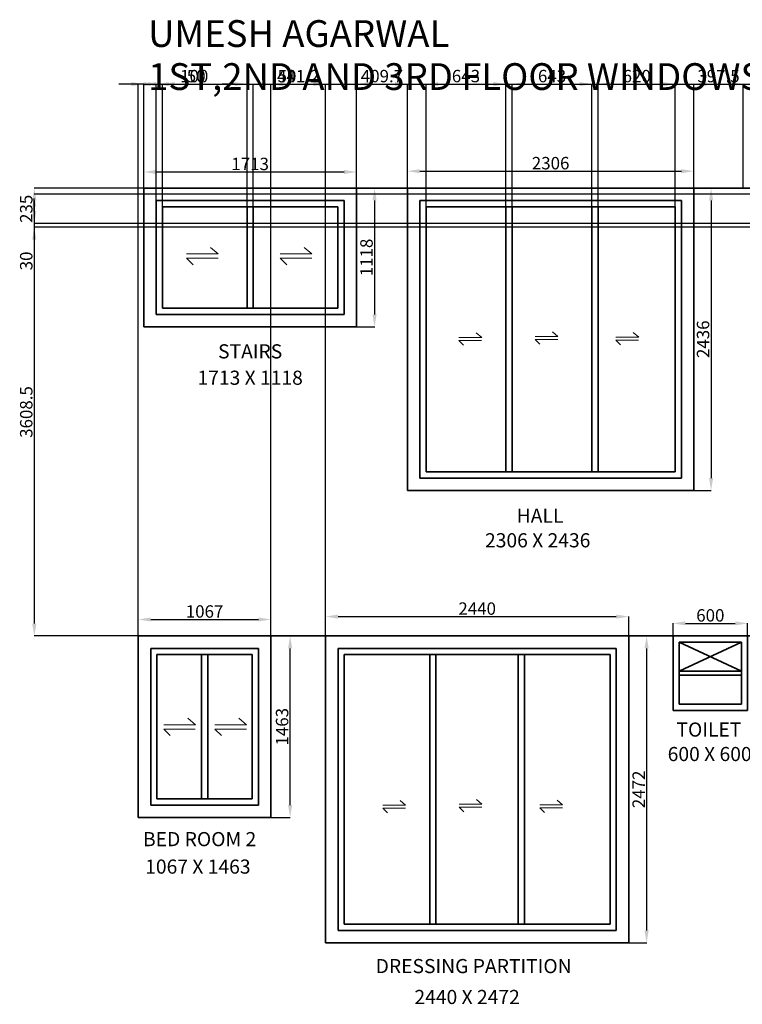
# Model space of a CAD drawing. Units: millimetres. Extents: x 5977 to 24120, y -1732 to 6209.
# Tile 1 of 3: x 5977 to 11795, y -1724 to 6209. Entities that reach past the tile are written whole.
import ezdxf

# ---------------------------------------------------------------- set-up
doc = ezdxf.new("R2010")
doc.units = ezdxf.units.MM
for name, color, linetype, lineweight in [('A-ANNO-DIMS', 2, 'Continuous', 18), ('A-ANNO-SYMB', 143, 'Continuous', 18), ('A-ANNO-TEXT', 7, 'Continuous', 25), ('A-GLAZ', 4, 'Continuous', 35)]:
    doc.layers.add(name, color=color, linetype=linetype, lineweight=lineweight)
doc.styles.get("Standard").update_dxf_attribs({"font": 'arial.ttf'})
doc.dimstyles.new('ISO-25', dxfattribs={"dimtxt": 100, "dimasz": 100, "dimexe": 1.25, "dimexo": 0.625, "dimtad": 1, "dimtxsty": 'Standard', "dimcen": 2.5, "dimadec": 0, "dimazin": 0, "dimtfac": 1, "dimtmove": 0, "dimatfit": 3, "dimfxl": 1, "dimarcsym": 0})

# ---------------------------------------------------------------- blocks, each defined once
blk = doc.blocks.new('*D1')
at = {"layer": 'A-ANNO-DIMS', "color": 0, "lineweight": -2, "transparency": 16777216}
for p, q in [((6975.8, 4852.8), (6975.8, 4983.1)), ((7075.8, 4981.9), (8588.8, 4981.9)), ((8688.8, 4852.8), (8688.8, 4983.1))]:
    blk.add_line(p, q, dxfattribs=at)
at = {"layer": 'A-ANNO-DIMS', "color": 0, "transparency": 16777216}
for points in [[(7075.8, 4998.5), (7075.8, 4965.2), (6975.8, 4981.9)], [(8588.8, 4998.5), (8588.8, 4965.2), (8688.8, 4981.9)]]:
    blk.add_solid(points, dxfattribs=at)
at = {"layer": 'Defpoints', "color": 0, "transparency": 16777216}
for p in [(8688.8, 4981.9), (6975.8, 4852.2), (8688.8, 4852.2)]:
    blk.add_point(p, dxfattribs=at)
at = {"layer": 'A-ANNO-DIMS', "color": 0, "transparency": 16777216, "insert": (7832.3, 5033.6), "char_height": 100, "attachment_point": 5}
blk.add_mtext('1713', dxfattribs=at)
blk = doc.blocks.new('*D2')
at = {"layer": 'A-ANNO-DIMS', "color": 0, "lineweight": -2, "transparency": 16777216}
for p, q in [((8689.4, 4852.2), (8835.1, 4852.2)), ((8833.9, 4752.2), (8833.9, 3834.2)), ((8689.4, 3734.2), (8835.1, 3734.2))]:
    blk.add_line(p, q, dxfattribs=at)
at = {"layer": 'A-ANNO-DIMS', "color": 0, "transparency": 16777216}
for points in [[(8817.2, 4752.2), (8850.5, 4752.2), (8833.9, 4852.2)], [(8817.2, 3834.2), (8850.5, 3834.2), (8833.9, 3734.2)]]:
    blk.add_solid(points, dxfattribs=at)
at = {"layer": 'Defpoints', "color": 0, "transparency": 16777216}
for p in [(8688.8, 4852.2), (8688.8, 3734.2), (8833.9, 3734.2)]:
    blk.add_point(p, dxfattribs=at)
at = {"layer": 'A-ANNO-DIMS', "color": 0, "transparency": 16777216, "insert": (8782.2, 4293.2), "char_height": 100, "attachment_point": 5, "rotation": 90}
blk.add_mtext('1118', dxfattribs=at)
blk = doc.blocks.new('*D3')
at = {"layer": 'A-ANNO-DIMS', "color": 0, "lineweight": -2, "transparency": 16777216}
for p, q in [((9098.5, 4852.8), (9098.5, 4989.4)), ((9198.5, 4988.2), (11304.5, 4988.2)), ((11404.5, 4852.8), (11404.5, 4989.4))]:
    blk.add_line(p, q, dxfattribs=at)
at = {"layer": 'A-ANNO-DIMS', "color": 0, "transparency": 16777216}
for points in [[(9198.5, 5004.8), (9198.5, 4971.5), (9098.5, 4988.2)], [(11304.5, 5004.8), (11304.5, 4971.5), (11404.5, 4988.2)]]:
    blk.add_solid(points, dxfattribs=at)
at = {"layer": 'Defpoints', "color": 0, "transparency": 16777216}
for p in [(11404.5, 4988.2), (9098.5, 4852.2), (11404.5, 4852.2)]:
    blk.add_point(p, dxfattribs=at)
at = {"layer": 'A-ANNO-DIMS', "color": 0, "transparency": 16777216, "insert": (10251.5, 5039.9), "char_height": 100, "attachment_point": 5}
blk.add_mtext('2306', dxfattribs=at)
blk = doc.blocks.new('*D4')
at = {"layer": 'A-ANNO-DIMS', "color": 0, "lineweight": -2, "transparency": 16777216}
for p, q in [((11405.1, 4852.2), (11544.6, 4852.2)), ((11543.4, 4752.2), (11543.4, 2516.2)), ((11405.1, 2416.2), (11544.6, 2416.2))]:
    blk.add_line(p, q, dxfattribs=at)
at = {"layer": 'A-ANNO-DIMS', "color": 0, "transparency": 16777216}
for points in [[(11526.7, 4752.2), (11560, 4752.2), (11543.4, 4852.2)], [(11526.7, 2516.2), (11560, 2516.2), (11543.4, 2416.2)]]:
    blk.add_solid(points, dxfattribs=at)
at = {"layer": 'Defpoints', "color": 0, "transparency": 16777216}
for p in [(11404.5, 4852.2), (11404.5, 2416.2), (11543.4, 2416.2)]:
    blk.add_point(p, dxfattribs=at)
at = {"layer": 'A-ANNO-DIMS', "color": 0, "transparency": 16777216, "insert": (11491.7, 3634.2), "char_height": 100, "attachment_point": 5, "rotation": 90}
blk.add_mtext('2436', dxfattribs=at)
blk = doc.blocks.new('*D21')
at = {"layer": 'A-ANNO-DIMS', "color": 0, "lineweight": -2, "transparency": 16777216}
for p, q in [((6931.9, 1244.3), (6931.9, 1377.5)), ((7031.9, 1376.2), (7898.9, 1376.2)), ((7998.9, 1244.3), (7998.9, 1377.5))]:
    blk.add_line(p, q, dxfattribs=at)
at = {"layer": 'A-ANNO-DIMS', "color": 0, "transparency": 16777216}
for points in [[(7031.9, 1392.9), (7031.9, 1359.6), (6931.9, 1376.2)], [(7898.9, 1392.9), (7898.9, 1359.6), (7998.9, 1376.2)]]:
    blk.add_solid(points, dxfattribs=at)
at = {"layer": 'Defpoints', "color": 0, "transparency": 16777216}
for p in [(7998.9, 1376.2), (6931.9, 1243.7), (7998.9, 1243.7)]:
    blk.add_point(p, dxfattribs=at)
at = {"layer": 'A-ANNO-DIMS', "color": 0, "transparency": 16777216, "insert": (7465.4, 1427.9), "char_height": 100, "attachment_point": 5}
blk.add_mtext('1067', dxfattribs=at)
blk = doc.blocks.new('*D22')
at = {"layer": 'A-ANNO-DIMS', "color": 0, "lineweight": -2, "transparency": 16777216}
for p, q in [((7999.6, 1243.7), (8155.6, 1243.7)), ((8154.3, -119.3), (8154.3, 1143.7)), ((7999.6, -219.3), (8155.6, -219.3))]:
    blk.add_line(p, q, dxfattribs=at)
at = {"layer": 'A-ANNO-DIMS', "color": 0, "transparency": 16777216}
for points in [[(8137.6, 1143.7), (8171, 1143.7), (8154.3, 1243.7)], [(8137.6, -119.3), (8171, -119.3), (8154.3, -219.3)]]:
    blk.add_solid(points, dxfattribs=at)
at = {"layer": 'Defpoints', "color": 0, "transparency": 16777216}
for p in [(7998.9, 1243.7), (8154.3, 1243.7), (7998.9, -219.3)]:
    blk.add_point(p, dxfattribs=at)
at = {"layer": 'A-ANNO-DIMS', "color": 0, "transparency": 16777216, "insert": (8102.6, 512.2), "char_height": 100, "attachment_point": 5, "rotation": 90}
blk.add_mtext('1463', dxfattribs=at)
blk = doc.blocks.new('*D23')
at = {"layer": 'A-ANNO-DIMS', "color": 0, "lineweight": -2, "transparency": 16777216}
for p, q in [((8440.1, 1244.3), (8440.1, 1400.7)), ((8540.1, 1399.4), (10780.1, 1399.4)), ((10880.1, 1244.3), (10880.1, 1400.7))]:
    blk.add_line(p, q, dxfattribs=at)
at = {"layer": 'A-ANNO-DIMS', "color": 0, "transparency": 16777216}
for points in [[(8540.1, 1416.1), (8540.1, 1382.7), (8440.1, 1399.4)], [(10780.1, 1416.1), (10780.1, 1382.7), (10880.1, 1399.4)]]:
    blk.add_solid(points, dxfattribs=at)
at = {"layer": 'Defpoints', "color": 0, "transparency": 16777216}
for p in [(10880.1, 1399.4), (8440.1, 1243.7), (10880.1, 1243.7)]:
    blk.add_point(p, dxfattribs=at)
at = {"layer": 'A-ANNO-DIMS', "color": 0, "transparency": 16777216, "insert": (9660.1, 1451.1), "char_height": 100, "attachment_point": 5}
blk.add_mtext('2440', dxfattribs=at)
blk = doc.blocks.new('*D24')
at = {"layer": 'A-ANNO-DIMS', "color": 0, "lineweight": -2, "transparency": 16777216}
for p, q in [((10880.7, 1243.7), (11025.5, 1243.7)), ((11024.2, 1143.7), (11024.2, -1128.3)), ((10880.7, -1228.3), (11025.5, -1228.3))]:
    blk.add_line(p, q, dxfattribs=at)
at = {"layer": 'A-ANNO-DIMS', "color": 0, "transparency": 16777216}
for points in [[(11007.5, 1143.7), (11040.9, 1143.7), (11024.2, 1243.7)], [(11007.5, -1128.3), (11040.9, -1128.3), (11024.2, -1228.3)]]:
    blk.add_solid(points, dxfattribs=at)
at = {"layer": 'Defpoints', "color": 0, "transparency": 16777216}
for p in [(10880.1, 1243.7), (10880.1, -1228.3), (11024.2, -1228.3)]:
    blk.add_point(p, dxfattribs=at)
at = {"layer": 'A-ANNO-DIMS', "color": 0, "transparency": 16777216, "insert": (10973.4, 7.7), "char_height": 100, "attachment_point": 5, "rotation": 90}
blk.add_mtext('2472', dxfattribs=at)
blk = doc.blocks.new('*D27')
at = {"layer": 'A-ANNO-DIMS', "color": 0, "lineweight": -2, "transparency": 16777216}
for p, q in [((11237.4, 1244.3), (11237.4, 1346.1)), ((11337.4, 1344.9), (11737.4, 1344.9)), ((11837.4, 1244.3), (11837.4, 1346.1))]:
    blk.add_line(p, q, dxfattribs=at)
at = {"layer": 'A-ANNO-DIMS', "color": 0, "transparency": 16777216}
for points in [[(11337.4, 1361.5), (11337.4, 1328.2), (11237.4, 1344.9)], [(11737.4, 1361.5), (11737.4, 1328.2), (11837.4, 1344.9)]]:
    blk.add_solid(points, dxfattribs=at)
at = {"layer": 'Defpoints', "color": 0, "transparency": 16777216}
for p in [(11837.4, 1344.9), (11237.4, 1243.7), (11837.4, 1243.7)]:
    blk.add_point(p, dxfattribs=at)
at = {"layer": 'A-ANNO-DIMS', "color": 0, "transparency": 16777216, "insert": (11537.4, 1396.6), "char_height": 100, "attachment_point": 5}
blk.add_mtext('600', dxfattribs=at)
blk = doc.blocks.new('WIN-600x600-TOILET')
for p, q in [((16540.9, 4852.2), (16540.9, 4252.2)), ((17140.9, 4252.2), (17140.9, 4852.2)), ((16590.9, 4802.2), (16590.9, 4302.2)), ((16590.9, 4802.2), (17090.9, 4802.2)), ((16590.9, 4567.2), (17090.9, 4802.2)), ((17090.9, 4567.2), (16590.9, 4802.2)), ((17090.9, 4302.2), (17090.9, 4802.2)), ((16590.9, 4567.2), (17090.9, 4567.2)), ((16590.9, 4302.2), (17090.9, 4302.2)), ((16540.9, 4252.2), (17140.9, 4252.2))]:
    blk.add_line(p, q)
blk = doc.blocks.new('ARROW-SLIDE')
for p, q in [((14721.8, 21.3), (14904.6, 21.3)), ((14904.6, 21.3), (14860.5, 58.6)), ((14721.8, -3.8), (14904.1, -3.8)), ((14721.8, -3.8), (14759.4, -41.4))]:
    blk.add_line(p, q)
blk = doc.blocks.new('ARROW-SLIDE-LG')
for p, q in [((7575.1, 4322.2), (7513.8, 4374)), ((7321, 4287.2), (7574.5, 4287.2)), ((7321, 4287.2), (7373.4, 4234.9)), ((7321.1, 4322.2), (7575.1, 4322.2))]:
    blk.add_line(p, q)
blk = doc.blocks.new('*D41')
at = {"layer": 'A-ANNO-DIMS', "color": 0, "lineweight": -2, "transparency": 16777216}
for p, q in [((6975.8, 4852.8), (6975.8, 5690.9)), ((7075.8, 5689.7), (23502.6, 5689.7)), ((23602.6, 4852.8), (23602.6, 5690.9))]:
    blk.add_line(p, q, dxfattribs=at)
at = {"layer": 'A-ANNO-DIMS', "color": 0, "transparency": 16777216}
for points in [[(7075.8, 5706.3), (7075.8, 5673), (6975.8, 5689.7)], [(23502.6, 5706.3), (23502.6, 5673), (23602.6, 5689.7)]]:
    blk.add_solid(points, dxfattribs=at)
at = {"layer": 'Defpoints', "color": 0, "transparency": 16777216}
for p in [(23602.6, 5689.7), (6975.8, 4852.2), (23602.6, 4852.2)]:
    blk.add_point(p, dxfattribs=at)
at = {"layer": 'A-ANNO-DIMS', "color": 0, "transparency": 16777216, "insert": (15289.2, 5741.3), "char_height": 100, "attachment_point": 5}
blk.add_mtext('16627', dxfattribs=at)
blk = doc.blocks.new('*D42')
at = {"layer": 'A-ANNO-DIMS', "color": 0, "lineweight": -2, "transparency": 16777216}
for p, q in [((6931.9, 1244.3), (6931.9, 5690.9)), ((7031.9, 5689.7), (20409.7, 5689.7)), ((20509.7, 1244.3), (20509.7, 5690.9))]:
    blk.add_line(p, q, dxfattribs=at)
at = {"layer": 'A-ANNO-DIMS', "color": 0, "transparency": 16777216}
for points in [[(7031.9, 5706.3), (7031.9, 5673), (6931.9, 5689.7)], [(20409.7, 5706.3), (20409.7, 5673), (20509.7, 5689.7)]]:
    blk.add_solid(points, dxfattribs=at)
at = {"layer": 'Defpoints', "color": 0, "transparency": 16777216}
for p in [(20509.7, 5689.7), (6931.9, 1243.7), (20509.7, 1243.7)]:
    blk.add_point(p, dxfattribs=at)
at = {"layer": 'A-ANNO-DIMS', "color": 0, "transparency": 16777216, "insert": (13720.8, 5741.4), "char_height": 100, "attachment_point": 5}
blk.add_mtext('13578', dxfattribs=at)
blk = doc.blocks.new('*D43')
at = {"layer": 'A-ANNO-DIMS', "color": 0, "lineweight": -2, "transparency": 16777216}
for p, q in [((6975.1, 4852.2), (6093.2, 4852.2)), ((6094.4, 4752.2), (6094.4, 1343.7)), ((6931.3, 1243.7), (6093.2, 1243.7))]:
    blk.add_line(p, q, dxfattribs=at)
at = {"layer": 'A-ANNO-DIMS', "color": 0, "transparency": 16777216}
for points in [[(6077.8, 4752.2), (6111.1, 4752.2), (6094.4, 4852.2)], [(6077.8, 1343.7), (6111.1, 1343.7), (6094.4, 1243.7)]]:
    blk.add_solid(points, dxfattribs=at)
at = {"layer": 'Defpoints', "color": 0, "transparency": 16777216}
for p in [(6975.8, 4852.2), (6094.4, 1243.7), (6931.9, 1243.7)]:
    blk.add_point(p, dxfattribs=at)
at = {"layer": 'A-ANNO-DIMS', "color": 0, "transparency": 16777216, "insert": (6042.7, 3047.9), "char_height": 100, "attachment_point": 5, "rotation": 90}
blk.add_mtext('3608.5', dxfattribs=at)
blk = doc.blocks.new('*D44')
at = {"layer": 'A-ANNO-DIMS', "color": 0, "lineweight": -2, "transparency": 16777216}
for p, q in [((8688.8, 4852.8), (8688.8, 5690.9)), ((8788.8, 5689.7), (8998.5, 5689.7)), ((9098.5, 4852.8), (9098.5, 5690.9))]:
    blk.add_line(p, q, dxfattribs=at)
at = {"layer": 'A-ANNO-DIMS', "color": 0, "transparency": 16777216}
for points in [[(8788.8, 5706.3), (8788.8, 5673), (8688.8, 5689.7)], [(8998.5, 5706.3), (8998.5, 5673), (9098.5, 5689.7)]]:
    blk.add_solid(points, dxfattribs=at)
at = {"layer": 'Defpoints', "color": 0, "transparency": 16777216}
for p in [(9098.5, 5689.7), (8688.8, 4852.2), (9098.5, 4852.2)]:
    blk.add_point(p, dxfattribs=at)
at = {"layer": 'A-ANNO-DIMS', "color": 0, "transparency": 16777216, "insert": (8893.6, 5741.3), "char_height": 100, "attachment_point": 5}
blk.add_mtext('409.7', dxfattribs=at)
blk = doc.blocks.new('*D45')
at = {"layer": 'A-ANNO-DIMS', "color": 0, "lineweight": -2, "transparency": 16777216}
for p, q in [((11404.5, 4852.8), (11404.5, 5690.9)), ((11504.5, 5689.7), (11702, 5689.7)), ((11802, 4852.8), (11802, 5690.9))]:
    blk.add_line(p, q, dxfattribs=at)
at = {"layer": 'A-ANNO-DIMS', "color": 0, "transparency": 16777216}
for points in [[(11504.5, 5706.3), (11504.5, 5673), (11404.5, 5689.7)], [(11702, 5706.3), (11702, 5673), (11802, 5689.7)]]:
    blk.add_solid(points, dxfattribs=at)
at = {"layer": 'Defpoints', "color": 0, "transparency": 16777216}
for p in [(11802, 5689.7), (11404.5, 4852.2), (11802, 4852.2)]:
    blk.add_point(p, dxfattribs=at)
at = {"layer": 'A-ANNO-DIMS', "color": 0, "transparency": 16777216, "insert": (11603.2, 5741.4), "char_height": 100, "attachment_point": 5}
blk.add_mtext('397.5', dxfattribs=at)
blk = doc.blocks.new('*D54')
at = {"layer": 'A-ANNO-DIMS', "color": 0, "lineweight": -2, "transparency": 16777216}
for p, q in [((7998.9, 1244.3), (7998.9, 5690.9)), ((8098.9, 5689.7), (8340.1, 5689.7)), ((8440.1, 1244.3), (8440.1, 5690.9))]:
    blk.add_line(p, q, dxfattribs=at)
at = {"layer": 'A-ANNO-DIMS', "color": 0, "transparency": 16777216}
for points in [[(8098.9, 5706.3), (8098.9, 5673), (7998.9, 5689.7)], [(8340.1, 5706.3), (8340.1, 5673), (8440.1, 5689.7)]]:
    blk.add_solid(points, dxfattribs=at)
at = {"layer": 'Defpoints', "color": 0, "transparency": 16777216}
for p in [(8440.1, 5689.7), (7998.9, 1243.7), (8440.1, 1243.7)]:
    blk.add_point(p, dxfattribs=at)
at = {"layer": 'A-ANNO-DIMS', "color": 0, "transparency": 16777216, "insert": (8219.5, 5740.5), "char_height": 100, "attachment_point": 5}
blk.add_mtext('441.2', dxfattribs=at)
blk = doc.blocks.new('*D61')
at = {"layer": 'A-ANNO-DIMS', "color": 0, "lineweight": -2, "transparency": 16777216}
for p, q in [((6875.8, 5689.7), (6775.8, 5689.7)), ((6975.8, 4852.8), (6975.8, 5690.9)), ((6975.8, 5689.7), (7075.8, 5689.7)), ((7075.8, 4752.8), (7075.8, 5690.9)), ((7175.8, 5689.7), (7488.2, 5689.7))]:
    blk.add_line(p, q, dxfattribs=at)
at = {"layer": 'A-ANNO-DIMS', "color": 0, "transparency": 16777216}
for points in [[(6875.8, 5706.3), (6875.8, 5673), (6975.8, 5689.7)], [(7175.8, 5706.3), (7175.8, 5673), (7075.8, 5689.7)]]:
    blk.add_solid(points, dxfattribs=at)
at = {"layer": 'Defpoints', "color": 0, "transparency": 16777216}
for p in [(7075.8, 5689.7), (6975.8, 4852.2), (7075.8, 4752.2)]:
    blk.add_point(p, dxfattribs=at)
at = {"layer": 'A-ANNO-DIMS', "color": 0, "transparency": 16777216, "insert": (7382, 5741.3), "char_height": 100, "attachment_point": 5}
blk.add_mtext('100', dxfattribs=at)
blk = doc.blocks.new('*D62')
at = {"layer": 'A-ANNO-DIMS', "color": 0, "lineweight": -2, "transparency": 16777216}
for p, q in [((6975.8, 5689.7), (6875.8, 5689.7)), ((7075.8, 4752.8), (7075.8, 5690.9)), ((7075.8, 5689.7), (7125.8, 5689.7)), ((7125.8, 4702.8), (7125.8, 5690.9)), ((7225.8, 5689.7), (7469.9, 5689.7))]:
    blk.add_line(p, q, dxfattribs=at)
at = {"layer": 'A-ANNO-DIMS', "color": 0, "transparency": 16777216}
for points in [[(6975.8, 5706.3), (6975.8, 5673), (7075.8, 5689.7)], [(7225.8, 5706.3), (7225.8, 5673), (7125.8, 5689.7)]]:
    blk.add_solid(points, dxfattribs=at)
at = {"layer": 'Defpoints', "color": 0, "transparency": 16777216}
for p in [(7125.8, 5689.7), (7075.8, 4752.2), (7125.8, 4702.2)]:
    blk.add_point(p, dxfattribs=at)
at = {"layer": 'A-ANNO-DIMS', "color": 0, "transparency": 16777216, "insert": (7397.8, 5741.3), "char_height": 100, "attachment_point": 5}
blk.add_mtext('50', dxfattribs=at)
blk = doc.blocks.new('*D63')
at = {"layer": 'A-ANNO-DIMS', "color": 0, "lineweight": -2, "transparency": 16777216}
for p, q in [((7707.3, 5689.7), (7607.3, 5689.7)), ((7807.3, 4702.8), (7807.3, 5690.9)), ((7807.3, 5689.7), (7857.3, 5689.7)), ((7857.3, 4702.8), (7857.3, 5690.9)), ((7957.3, 5689.7), (8201.4, 5689.7))]:
    blk.add_line(p, q, dxfattribs=at)
at = {"layer": 'A-ANNO-DIMS', "color": 0, "transparency": 16777216}
for points in [[(7707.3, 5706.3), (7707.3, 5673), (7807.3, 5689.7)], [(7957.3, 5706.3), (7957.3, 5673), (7857.3, 5689.7)]]:
    blk.add_solid(points, dxfattribs=at)
at = {"layer": 'Defpoints', "color": 0, "transparency": 16777216}
for p in [(7857.3, 5689.7), (7807.3, 4702.2), (7857.3, 4702.2)]:
    blk.add_point(p, dxfattribs=at)
at = {"layer": 'A-ANNO-DIMS', "color": 0, "transparency": 16777216, "insert": (8129.3, 5741.3), "char_height": 100, "attachment_point": 5}
blk.add_mtext('50', dxfattribs=at)
blk = doc.blocks.new('*D64')
at = {"layer": 'A-ANNO-DIMS', "color": 0, "lineweight": -2, "transparency": 16777216}
for p, q in [((9248.5, 4702.8), (9248.5, 5690.9)), ((9348.5, 5689.7), (9791.5, 5689.7)), ((9891.5, 4702.8), (9891.5, 5690.9))]:
    blk.add_line(p, q, dxfattribs=at)
at = {"layer": 'A-ANNO-DIMS', "color": 0, "transparency": 16777216}
for points in [[(9348.5, 5706.3), (9348.5, 5673), (9248.5, 5689.7)], [(9791.5, 5706.3), (9791.5, 5673), (9891.5, 5689.7)]]:
    blk.add_solid(points, dxfattribs=at)
at = {"layer": 'Defpoints', "color": 0, "transparency": 16777216}
for p in [(9891.5, 5689.7), (9248.5, 4702.2), (9891.5, 4702.2)]:
    blk.add_point(p, dxfattribs=at)
at = {"layer": 'A-ANNO-DIMS', "color": 0, "transparency": 16777216, "insert": (9570, 5741.4), "char_height": 100, "attachment_point": 5}
blk.add_mtext('643', dxfattribs=at)
blk = doc.blocks.new('*D65')
at = {"layer": 'A-ANNO-DIMS', "color": 0, "lineweight": -2, "transparency": 16777216}
for p, q in [((9941.5, 4702.8), (9941.5, 5690.9)), ((10041.5, 5689.7), (10484.5, 5689.7)), ((10584.5, 4702.8), (10584.5, 5690.9))]:
    blk.add_line(p, q, dxfattribs=at)
at = {"layer": 'A-ANNO-DIMS', "color": 0, "transparency": 16777216}
for points in [[(10041.5, 5706.3), (10041.5, 5673), (9941.5, 5689.7)], [(10484.5, 5706.3), (10484.5, 5673), (10584.5, 5689.7)]]:
    blk.add_solid(points, dxfattribs=at)
at = {"layer": 'Defpoints', "color": 0, "transparency": 16777216}
for p in [(10584.5, 5689.7), (9941.5, 4702.2), (10584.5, 4702.2)]:
    blk.add_point(p, dxfattribs=at)
at = {"layer": 'A-ANNO-DIMS', "color": 0, "transparency": 16777216, "insert": (10263, 5741.4), "char_height": 100, "attachment_point": 5}
blk.add_mtext('643', dxfattribs=at)
blk = doc.blocks.new('*D66')
at = {"layer": 'A-ANNO-DIMS', "color": 0, "lineweight": -2, "transparency": 16777216}
for p, q in [((10634.5, 4702.8), (10634.5, 5690.9)), ((10734.5, 5689.7), (11154.5, 5689.7)), ((11254.5, 4702.8), (11254.5, 5690.9))]:
    blk.add_line(p, q, dxfattribs=at)
at = {"layer": 'A-ANNO-DIMS', "color": 0, "transparency": 16777216}
for points in [[(10734.5, 5706.3), (10734.5, 5673), (10634.5, 5689.7)], [(11154.5, 5706.3), (11154.5, 5673), (11254.5, 5689.7)]]:
    blk.add_solid(points, dxfattribs=at)
at = {"layer": 'Defpoints', "color": 0, "transparency": 16777216}
for p in [(11254.5, 5689.7), (10634.5, 4702.2), (11254.5, 4702.2)]:
    blk.add_point(p, dxfattribs=at)
at = {"layer": 'A-ANNO-DIMS', "color": 0, "transparency": 16777216, "insert": (10944.5, 5741.3), "char_height": 100, "attachment_point": 5}
blk.add_mtext('620', dxfattribs=at)
blk = doc.blocks.new('*D67')
at = {"layer": 'A-ANNO-DIMS', "color": 0, "lineweight": -2, "transparency": 16777216}
for p, q in [((16590.3, 4802.2), (6093.2, 4802.2)), ((6094.4, 4702.2), (6094.4, 4667.2)), ((16590.3, 4567.2), (6093.2, 4567.2))]:
    blk.add_line(p, q, dxfattribs=at)
at = {"layer": 'A-ANNO-DIMS', "color": 0, "transparency": 16777216}
for points in [[(6077.8, 4702.2), (6111.1, 4702.2), (6094.4, 4802.2)], [(6077.8, 4667.2), (6111.1, 4667.2), (6094.4, 4567.2)]]:
    blk.add_solid(points, dxfattribs=at)
at = {"layer": 'Defpoints', "color": 0, "transparency": 16777216}
for p in [(16590.9, 4802.2), (6094.4, 4567.2), (16590.9, 4567.2)]:
    blk.add_point(p, dxfattribs=at)
at = {"layer": 'A-ANNO-DIMS', "color": 0, "transparency": 16777216, "insert": (6042.7, 4684.7), "char_height": 100, "attachment_point": 5, "rotation": 90}
blk.add_mtext('235', dxfattribs=at)
blk = doc.blocks.new('*D68')
at = {"layer": 'A-ANNO-DIMS', "color": 0, "lineweight": -2, "transparency": 16777216}
for p, q in [((6094.4, 4667.2), (6094.4, 4767.2)), ((16590.3, 4567.2), (6093.2, 4567.2)), ((16590.3, 4537.2), (6093.2, 4537.2)), ((6094.4, 4567.2), (6094.4, 4537.2)), ((6094.4, 4437.2), (6094.4, 4193.1))]:
    blk.add_line(p, q, dxfattribs=at)
at = {"layer": 'A-ANNO-DIMS', "color": 0, "transparency": 16777216}
for points in [[(6077.8, 4667.2), (6111.1, 4667.2), (6094.4, 4567.2)], [(6077.8, 4437.2), (6111.1, 4437.2), (6094.4, 4537.2)]]:
    blk.add_solid(points, dxfattribs=at)
at = {"layer": 'Defpoints', "color": 0, "transparency": 16777216}
for p in [(6094.4, 4537.2), (16590.9, 4567.2), (16590.9, 4537.2)]:
    blk.add_point(p, dxfattribs=at)
at = {"layer": 'A-ANNO-DIMS', "color": 0, "transparency": 16777216, "insert": (6042.7, 4265.1), "char_height": 100, "attachment_point": 5, "rotation": 90}
blk.add_mtext('30', dxfattribs=at)

msp = doc.modelspace()

# ---------------------------------------------------------------- linework, layer by layer
at = {"layer": 'A-GLAZ'}
for p, q in [((8688.757, 4852.16), (6975.757, 4852.16)), ((6975.757, 4852.16), (6975.757, 3734.16)), ((6975.757, 4852.16), (19747.827, 4852.16)), ((8688.757, 3734.16), (8688.757, 4852.16)), ((9098.482, 4852.16), (9098.482, 2416.16)), ((11404.482, 2416.16), (11404.482, 4852.16)), ((7075.757, 4752.16), (8588.757, 4752.16)), ((7075.757, 4752.16), (7075.757, 3834.16)), ((7125.757, 4702.16), (7125.757, 3884.16)), ((7125.757, 4702.16), (8538.757, 4702.16)), ((7807.257, 4702.16), (7807.257, 3884.16)), ((7857.257, 4702.16), (7857.257, 3884.16)), ((8538.757, 3884.16), (8538.757, 4702.16)), ((8588.757, 3834.16), (8588.757, 4752.16)), ((9198.482, 4752.16), (9198.482, 2516.16)), ((9198.482, 4752.16), (11304.482, 4752.16)), ((9248.482, 4702.16), (9248.482, 2566.16)), ((9248.482, 4702.16), (11254.482, 4702.16)), ((9891.482, 4702.16), (9891.482, 2566.16)), ((9941.482, 4702.16), (9941.482, 2566.16)), ((10584.482, 4702.16), (10584.482, 2566.16)), ((10634.482, 4702.16), (10634.482, 2566.16)), ((11254.482, 2566.16), (11254.482, 4702.16)), ((11304.482, 2516.16), (11304.482, 4752.16)), ((7075.757, 3834.16), (8588.757, 3834.16)), ((7125.757, 3884.16), (8538.757, 3884.16)), ((6975.757, 3734.16), (8688.757, 3734.16)), ((9248.482, 2566.16), (11254.482, 2566.16)), ((9198.482, 2516.16), (11304.482, 2516.16)), ((9098.482, 2416.16), (11404.482, 2416.16)), ((6931.935, 1243.651), (20509.687, 1243.651)), ((6931.935, 1243.651), (6931.935, -219.349)), ((7998.935, -219.349), (7998.935, 1243.651)), ((8440.11, 1243.651), (8440.11, -1228.349)), ((10880.11, -1228.349), (10880.11, 1243.651)), ((7031.935, 1143.651), (7031.935, -119.349)), ((7031.935, 1143.651), (7898.935, 1143.651)), ((7898.935, -119.349), (7898.935, 1143.651)), ((8540.11, 1143.651), (10780.11, 1143.651)), ((8540.11, 1143.651), (8540.11, -1128.349)), ((10780.11, -1128.349), (10780.11, 1143.651)), ((7081.935, 1093.651), (7081.935, -69.349)), ((7081.935, 1093.651), (7848.935, 1093.651)), ((7440.435, -69.349), (7440.435, 1093.651)), ((7490.435, -69.349), (7490.435, 1093.651)), ((7848.935, -69.349), (7848.935, 1093.651)), ((8590.11, 1093.651), (10730.11, 1093.651)), ((8590.11, 1093.651), (8590.11, -1078.349)), ((9278.11, 1093.651), (9278.11, -1078.349)), ((9328.11, 1093.651), (9328.11, -1078.349)), ((9991.11, 1093.651), (9991.11, -1078.349)), ((10041.11, 1093.651), (10041.11, -1078.349)), ((10730.11, -1078.349), (10730.11, 1093.651)), ((11287.351, 928.651), (11787.351, 928.651)), ((7081.935, -69.349), (7848.935, -69.349)), ((7031.935, -119.349), (7898.935, -119.349)), ((6931.935, -219.349), (7998.935, -219.349)), ((8590.11, -1078.349), (10730.11, -1078.349)), ((8540.11, -1128.349), (10780.11, -1128.349)), ((8440.11, -1228.349), (10880.11, -1228.349))]:
    msp.add_line(p, q, dxfattribs=at)

# ---------------------------------------------------------------- block references
at = {"layer": 'A-ANNO-SYMB'}
for name, p in [('ARROW-SLIDE-LG', (0, 0)), ('ARROW-SLIDE-LG', (753.371, 0)), ('ARROW-SLIDE', (-5208.144, 3627.925)), ('ARROW-SLIDE', (-4594.266, 3635.135)), ('ARROW-SLIDE', (-3944.084, 3629.437)), ('ARROW-SLIDE-LG', (-183.985, -3793.877)), ('ARROW-SLIDE-LG', (227.771, -3793.877)), ('ARROW-SLIDE', (-5206.621, -132.484)), ('ARROW-SLIDE', (-5820.499, -139.693)), ('ARROW-SLIDE', (-4556.439, -138.181))]:
    msp.add_blockref(name, p, dxfattribs=at)
at = {"layer": 'A-GLAZ'}
msp.add_blockref('WIN-600x600-TOILET', (-5303.553, -3608.51), dxfattribs=at)

# ---------------------------------------------------------------- texts
at = {"layer": 'A-ANNO-TEXT'}
for s, height, p in [('UMESH AGARWAL', 215.75319, (7010.9, 5989.066)), ('1ST,2ND AND 3RD FLOOR WINDOWS', 215.75319, (7010.9, 5642.477)), ('STAIRS ', 113.8754, (7574.056, 3479.49)), ('1713 X 1118', 113.87539, (7408.339, 3267.186)), ('HALL ', 113.8754, (9978.218, 2155.241)), ('2306 X 2436', 113.87539, (9723.372, 1957.407)), ('TOILET', 113.8754, (11264.499, 432.677)), ('600 X 600', 113.8754, (11193.932, 235.504)), ('BED ROOM 2', 113.8754, (6969.814, -450.099)), ('1067 X 1463', 113.87539, (6987.347, -671.473)), ('DRESSING PARTITION', 113.87539, (8842.587, -1473.047)), ('2440 X 2472', 113.87539, (9155.016, -1722.004))]:
    msp.add_text(s, height=height, dxfattribs=at).set_placement(p)

# ---------------------------------------------------------------- dimensions: what is measured, and where the dimension line sits
at = {"layer": 'A-ANNO-DIMS'}
for base, p1, p2, override, picture, middle in [((7075.757, 5689.66), (6975.757, 4852.16), (7075.757, 4752.16), {"dimdec": 0, "dimlfac": 1, "dimrnd": 0, "dimzin": 0, "dimdsep": 46, "dimlunit": 2}, '*D61', (7381.975, 5741.343)), ((7125.757, 5689.66), (7075.757, 4752.16), (7125.757, 4702.16), {"dimdec": 0, "dimlfac": 1, "dimrnd": 0, "dimzin": 0, "dimdsep": 46, "dimlunit": 2}, '*D62', (7397.835, 5741.343)), ((20509.687, 5689.66), (6931.935, 1243.651), (20509.687, 1243.651), {"dimdec": 0, "dimlfac": 1, "dimrnd": 0, "dimzin": 0, "dimdsep": 46, "dimlunit": 2}, '*D42', (13720.811, 5741.377)), ((23602.612, 5689.66), (6975.757, 4852.16), (23602.612, 4852.16), {"dimdec": 0, "dimlfac": 1, "dimrnd": 0, "dimzin": 0, "dimdsep": 46, "dimlunit": 2}, '*D41', (15289.184, 5741.343)), ((7857.257, 5689.66), (7807.257, 4702.16), (7857.257, 4702.16), {"dimdec": 0, "dimlfac": 1, "dimrnd": 0, "dimzin": 0, "dimdsep": 46, "dimlunit": 2}, '*D63', (8129.335, 5741.343)), ((8440.11, 5689.66), (7998.935, 1243.651), (8440.11, 1243.651), {"dimdec": 1, "dimlfac": 1, "dimrnd": 0, "dimzin": 0, "dimdsep": 46, "dimlunit": 2}, '*D54', (8219.523, 5740.49)), ((9098.482, 5689.66), (8688.757, 4852.16), (9098.482, 4852.16), {"dimdec": 1, "dimlfac": 1, "dimrnd": 0, "dimzin": 0, "dimdsep": 46, "dimlunit": 2}, '*D44', (8893.619, 5741.343)), ((9891.482, 5689.66), (9248.482, 4702.16), (9891.482, 4702.16), {"dimdec": 0, "dimlfac": 1, "dimrnd": 0, "dimzin": 0, "dimdsep": 46, "dimlunit": 2}, '*D64', (9569.982, 5741.377)), ((10584.482, 5689.66), (9941.482, 4702.16), (10584.482, 4702.16), {"dimdec": 0, "dimlfac": 1, "dimrnd": 0, "dimzin": 0, "dimdsep": 46, "dimlunit": 2}, '*D65', (10262.982, 5741.377)), ((11254.482, 5689.66), (10634.482, 4702.16), (11254.482, 4702.16), {"dimdec": 0, "dimlfac": 1, "dimrnd": 0, "dimzin": 0, "dimdsep": 46, "dimlunit": 2}, '*D66', (10944.482, 5741.343)), ((11801.995, 5689.66), (11404.482, 4852.16), (11801.995, 4852.16), {"dimdec": 1, "dimlfac": 1, "dimrnd": 0, "dimzin": 0, "dimdsep": 46, "dimlunit": 2}, '*D45', (11603.238, 5741.377)), ((8688.757, 4981.878), (6975.757, 4852.16), (8688.757, 4852.16), {"dimclrd": 0, "dimclre": 0, "dimclrt": 0}, '*D1', (7832.257, 5033.594)), ((11404.482, 4988.157), (9098.482, 4852.16), (11404.482, 4852.16), {"dimclrd": 0, "dimclre": 0, "dimclrt": 0}, '*D3', (10251.482, 5039.873)), ((10880.11, 1399.407), (8440.11, 1243.651), (10880.11, 1243.651), {"dimclrd": 0, "dimclre": 0, "dimclrt": 0}, '*D23', (9660.11, 1451.089)), ((7998.935, 1376.225), (6931.935, 1243.651), (7998.935, 1243.651), {"dimclrd": 0, "dimclre": 0, "dimclrt": 0}, '*D21', (7465.435, 1427.908)), ((11837.351, 1344.88), (11237.351, 1243.651), (11837.351, 1243.651), {"dimclrd": 0, "dimclre": 0, "dimclrt": 0}, '*D27', (11537.351, 1396.562))]:
    dim = msp.add_linear_dim(base=base, p1=p1, p2=p2, dimstyle='ISO-25', override=override, dxfattribs=at)
    dim.commit()
    dim.dimension.update_dxf_attribs({"geometry": picture, "text_midpoint": middle})
for base, p1, p2, override, picture, middle in [((6094.435, 1243.651), (6975.757, 4852.16), (6931.935, 1243.651), {"dimdec": 1, "dimlfac": 1, "dimrnd": 0, "dimzin": 0, "dimdsep": 46, "dimlunit": 2}, '*D43', (6042.718, 3047.906)), ((8833.853, 3734.16), (8688.757, 4852.16), (8688.757, 3734.16), {"dimclrd": 0, "dimclre": 0, "dimclrt": 0}, '*D2', (8782.171, 4293.16)), ((11543.373, 2416.16), (11404.482, 4852.16), (11404.482, 2416.16), {"dimclrd": 0, "dimclre": 0, "dimclrt": 0}, '*D4', (11491.656, 3634.16)), ((6094.435, 4567.16), (16590.904, 4802.16), (16590.904, 4567.16), {"dimdec": 0, "dimlfac": 1, "dimrnd": 0, "dimzin": 0, "dimdsep": 46, "dimlunit": 2}, '*D67', (6042.718, 4684.66)), ((6094.435, 4537.16), (16590.904, 4567.16), (16590.904, 4537.16), {"dimdec": 0, "dimlfac": 1, "dimrnd": 0, "dimzin": 0, "dimdsep": 46, "dimlunit": 2}, '*D68', (6042.718, 4265.117)), ((8154.307, 1243.651), (7998.935, -219.349), (7998.935, 1243.651), {"dimclrd": 0, "dimclre": 0, "dimclrt": 0}, '*D22', (8102.59, 512.151))]:
    dim = msp.add_linear_dim(base=base, p1=p1, p2=p2, angle=90, dimstyle='ISO-25', override=override, dxfattribs=at)
    dim.commit()
    dim.dimension.update_dxf_attribs({"geometry": picture, "text_midpoint": middle})
dim = msp.add_linear_dim(base=(11024.211, -1228.349), p1=(10880.11, 1243.651), p2=(10880.11, -1228.349), angle=90, dimstyle='ISO-25', override={"dimclrd": 0, "dimclre": 0, "dimclrt": 0}, dxfattribs=at)
dim.commit()
dim.dimension.update_dxf_attribs({"geometry": '*D24', "text_midpoint": (11024.211, 7.651), "dimtype": 160})

doc.saveas('drawing.dxf')
